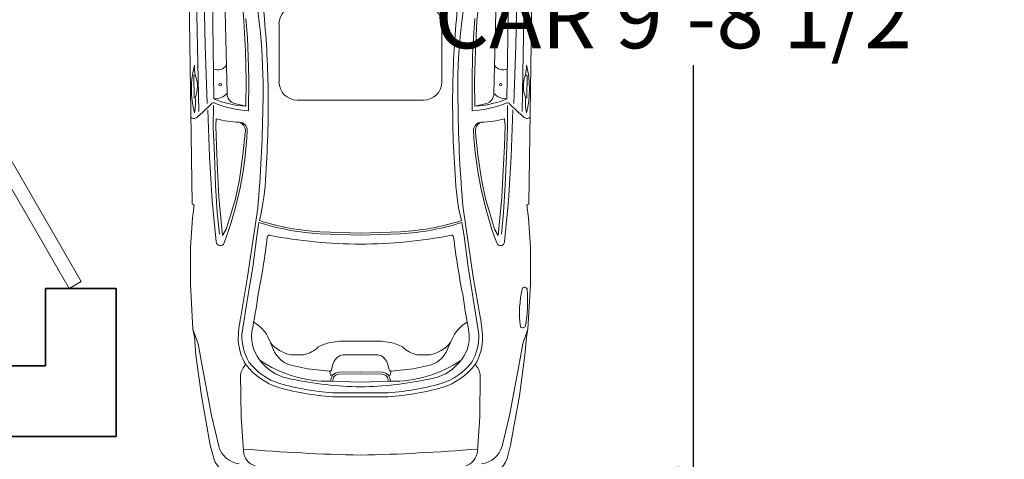
# Model space of a CAD drawing. Units: inches. Extents: x 2558 to 3026, y 433 to 1053.
# Tile 3 of 8: x 2795 to 2921, y 518 to 574. Entities that reach past the tile are written whole.
import ezdxf

# ---------------------------------------------------------------- set-up
doc = ezdxf.new("R2010")
doc.units = ezdxf.units.IN
for name, color, linetype, lineweight in [('0_Equip', 250, 'Continuous', 13), ('A-ANNO-DIMS', 2, 'Continuous', 18), ('A-DOOR', 4, 'Continuous', 18), ('A-WALL', 7, 'Continuous', 35)]:
    doc.layers.add(name, color=color, linetype=linetype, lineweight=lineweight)
doc.styles.get("Standard").update_dxf_attribs({"font": 'arial.ttf'})
doc.dimstyles.new('ISO-25', dxfattribs={"dimtxt": 8, "dimasz": 4, "dimexe": 1, "dimexo": 1, "dimgap": 1, "dimtad": 0, "dimtih": 1, "dimtoh": 1, "dimlunit": 3, "dimtxsty": 'Standard', "dimblk": 'OBLIQUE', "dimcen": 2.5, "dimclrt": 1, "dimadec": 0, "dimazin": 0, "dimtfac": 1, "dimtmove": 0, "dimatfit": 3, "dimfxl": 1, "dimfxlon": 1, "dimarcsym": 0})

# ---------------------------------------------------------------- blocks, each defined once
blk = doc.blocks.new('*U8')
for p, q in [((0, 0), (0, -6)), ((36, 0), (36, -6))]:
    blk.add_line(p, q)
blk.add_lwpolyline([(0, 0), (31.18, 18), (32.05, 16.48), (0.87, -1.52)], close=True)
blk.add_arc((0, 0), 36, 0, 30)
blk = doc.blocks.new('A$C4C7B54D1')
at = {"layer": '0_Equip', "ltscale": 0.1}
for p, q in [((-1.6171, 0.8152), (-1.5964, -0.6171)), ((-1.5805, 0.8299), (-1.5623, -0.138)), ((-1.4835, -0.0735), (-1.497, 0.863)), ((0.0322, -0.0735), (0.0457, 0.863)), ((0.1292, 0.8299), (0.111, -0.138)), ((0.1658, 0.8152), (0.145, -0.6171)), ((-1.4352, 0.792), (-1.4152, -0.045)), ((-0.0162, 0.792), (-0.0361, -0.045)), ((-1.5355, 0.484), (-1.5292, 0.2045)), ((0.0842, 0.484), (0.0779, 0.2045)), ((-1.3321, 0.3749), (-1.3286, 0.3301)), ((-0.1192, 0.3749), (-0.1228, 0.3301)), ((-1.3286, 0.3301), (-1.3204, 0.1751)), ((-1.3178, 0.3418), (-1.31, 0.2426)), ((-1.1468, 0.3145), (-1.1468, 0.0145)), ((-0.3045, 0.3145), (-0.3045, 0.0145)), ((-0.1335, 0.3418), (-0.1413, 0.2426)), ((-0.1228, 0.3301), (-0.1309, 0.1751)), ((-1.5292, 0.2045), (-1.5185, -0.0974)), ((-1.31, 0.2426), (-1.306, 0.1454)), ((-0.1413, 0.2426), (-0.1454, 0.1454)), ((0.0779, 0.2045), (0.0672, -0.0974)), ((-1.3204, 0.1751), (-1.3164, 0.0193)), ((-0.1309, 0.1751), (-0.1349, 0.0193)), ((-1.306, 0.1454), (-1.3036, 0.0305)), ((-0.1454, 0.1454), (-0.1478, 0.0305)), ((-1.5798, 0.0505), (-1.5879, 0.0456)), ((-1.5879, 0.0456), (-1.5863, -0.0676)), ((-1.3164, 0.0193), (-1.3178, -0.1112)), ((-1.3036, 0.0305), (-1.3044, -0.1358)), ((-0.1478, 0.0305), (-0.147, -0.1358)), ((-0.1349, 0.0193), (-0.1335, -0.1112)), ((0.1285, 0.0505), (0.1365, 0.0456)), ((0.1365, 0.0456), (0.1349, -0.0676)), ((-1.5863, -0.0676), (-1.5806, -0.0692)), ((-1.4948, -0.0965), (-1.5413, -0.143)), ((-1.3774, -0.0972), (-1.3178, -0.1112)), ((-0.7257, -0.0796), (-1.0528, -0.0796)), ((-0.7257, -0.0796), (-0.3986, -0.0796)), ((-0.0739, -0.0972), (-0.1335, -0.1112)), ((0.0435, -0.0965), (0.0899, -0.143)), ((0.1349, -0.0676), (0.1293, -0.0692)), ((-1.5413, -0.143), (-1.5686, -0.1663)), ((-1.5147, -0.1299), (-1.5058, -0.3725)), ((-1.4857, -0.1082), (-1.4866, -0.2223)), ((0.0344, -0.1082), (0.0352, -0.2223)), ((0.0633, -0.1299), (0.0545, -0.3725)), ((0.0899, -0.143), (0.1172, -0.1663)), ((-1.4713, -0.1773), (-1.4737, -0.2127)), ((0.02, -0.1773), (0.0224, -0.2127)), ((-1.4866, -0.2223), (-1.4809, -0.3653)), ((-1.4737, -0.2127), (-1.4705, -0.3187)), ((-1.3211, -0.2496), (-1.3332, -0.3629)), ((-0.1302, -0.2496), (-0.1182, -0.3629)), ((0.0224, -0.2127), (0.0192, -0.3187)), ((0.0352, -0.2223), (0.0296, -0.3653)), ((-1.4705, -0.3187), (-1.4649, -0.4424)), ((0.0192, -0.3187), (0.0135, -0.4424)), ((-1.5058, -0.3725), (-1.4922, -0.6007)), ((-1.4809, -0.3653), (-1.4745, -0.5203)), ((-1.3332, -0.3629), (-1.3516, -0.4906)), ((-0.1182, -0.3629), (-0.0997, -0.4906)), ((0.0296, -0.3653), (0.0232, -0.5203)), ((0.0545, -0.3725), (0.0408, -0.6007)), ((-1.4649, -0.4424), (-1.4576, -0.5822)), ((0.0135, -0.4424), (0.0063, -0.5822)), ((-1.3516, -0.4906), (-1.3725, -0.5902)), ((-0.0997, -0.4906), (-0.0788, -0.5902)), ((-1.4745, -0.5203), (-1.4665, -0.6617)), ((0.0232, -0.5203), (0.0151, -0.6617)), ((-1.4922, -0.6007), (-1.4712, -0.814)), ((-1.4576, -0.5822), (-1.4384, -0.7806)), ((-1.3725, -0.5902), (-1.3942, -0.6641)), ((-0.0788, -0.5902), (-0.0571, -0.6641)), ((0.0063, -0.5822), (-0.013, -0.7806)), ((0.0408, -0.6007), (0.0198, -0.814)), ((-1.5964, -0.6171), (-1.5863, -0.6228)), ((-1.5863, -0.6228), (-1.5949, -0.6885)), ((-1.4665, -0.6617), (-1.4552, -0.7742)), ((-1.3094, -0.9936), (-1.2569, -0.6398)), ((-0.1419, -0.9936), (-0.1944, -0.6398)), ((0.0151, -0.6617), (0.0039, -0.7742)), ((0.145, -0.6171), (0.1349, -0.6228)), ((0.1349, -0.6228), (0.1436, -0.6885)), ((-1.5949, -0.6885), (-1.605, -0.843)), ((-1.3942, -0.6641), (-1.4199, -0.7485)), ((-0.0571, -0.6641), (-0.0314, -0.7485)), ((0.1436, -0.6885), (0.1537, -0.843)), ((-1.4199, -0.7485), (-1.4384, -0.7806)), ((-1.2616, -0.7846), (-1.2511, -0.7134)), ((-0.9331, -0.7613), (-0.7253, -0.7683)), ((-0.5182, -0.7613), (-0.726, -0.7683)), ((-0.1898, -0.7846), (-0.2003, -0.7134)), ((-0.0314, -0.7485), (-0.013, -0.7806)), ((-1.2826, -0.9445), (-1.2616, -0.7846)), ((-0.9336, -0.7717), (-0.7257, -0.7787)), ((-0.5177, -0.7717), (-0.7257, -0.7787)), ((-0.1688, -0.9445), (-0.1898, -0.7846)), ((-1.605, -0.843), (-1.605, -1.0322)), ((0.1537, -0.843), (0.1537, -1.0322)), ((-1.3094, -1.1068), (-1.2826, -0.9445)), ((-0.1419, -1.1068), (-0.1688, -0.9445)), ((-1.3444, -1.2014), (-1.3094, -0.9936)), ((-0.1069, -1.2014), (-0.1419, -0.9936)), ((-1.605, -1.0322), (-1.592, -1.2661)), ((0.1537, -1.0322), (0.1407, -1.2661)), ((-1.3386, -1.2925), (-1.3094, -1.1068)), ((-0.1127, -1.2925), (-0.1419, -1.1068)), ((-1.565, -1.3405), (-1.592, -1.2661)), ((-1.592, -1.2661), (-1.5848, -1.3051)), ((0.1137, -1.3405), (0.1407, -1.2661)), ((0.1407, -1.2661), (0.1335, -1.3051)), ((-1.5848, -1.3051), (-1.5762, -1.4004)), ((-1.1985, -1.3182), (-1.1694, -1.3835)), ((-0.2528, -1.3182), (-0.282, -1.3835)), ((0.1335, -1.3051), (0.1248, -1.4004)), ((-1.5417, -1.4736), (-1.565, -1.3405)), ((-0.88, -1.3337), (-0.8328, -1.3271)), ((-0.8328, -1.3271), (-0.7257, -1.3271)), ((-0.6185, -1.3271), (-0.7257, -1.3271)), ((-0.5713, -1.3337), (-0.6185, -1.3271)), ((0.0904, -1.4736), (0.1137, -1.3405)), ((-1.5762, -1.4004), (-1.5486, -1.6107)), ((-1.0858, -1.3979), (-1.0181, -1.3979)), ((-0.8558, -1.4236), (-0.861, -1.4312)), ((-0.8488, -1.4158), (-0.8558, -1.4236)), ((-0.8409, -1.4088), (-0.8488, -1.4158)), ((-0.8309, -1.402), (-0.8409, -1.4088)), ((-0.8163, -1.3979), (-0.8309, -1.402)), ((-0.7257, -1.3974), (-0.8163, -1.3979)), ((-0.7257, -1.3974), (-0.635, -1.3979)), ((-0.635, -1.3979), (-0.6204, -1.402)), ((-0.6204, -1.402), (-0.6104, -1.4088)), ((-0.6104, -1.4088), (-0.6025, -1.4158)), ((-0.6025, -1.4158), (-0.5955, -1.4236)), ((-0.5955, -1.4236), (-0.5904, -1.4312)), ((-0.3655, -1.3979), (-0.4333, -1.3979)), ((0.1248, -1.4004), (0.0973, -1.6107)), ((-1.4962, -1.7129), (-1.5417, -1.4736)), ((-1.0923, -1.4501), (-0.9989, -1.4699)), ((-0.9989, -1.4699), (-0.8846, -1.4828)), ((-0.8745, -1.477), (-0.8769, -1.4791)), ((-0.8731, -1.467), (-0.8745, -1.477)), ((-0.8696, -1.4545), (-0.8731, -1.467)), ((-0.8664, -1.4423), (-0.8696, -1.4545)), ((-0.861, -1.4312), (-0.8664, -1.4423)), ((-0.5904, -1.4312), (-0.585, -1.4423)), ((-0.585, -1.4423), (-0.5817, -1.4545)), ((-0.5817, -1.4545), (-0.5782, -1.467)), ((-0.5782, -1.467), (-0.5768, -1.477)), ((-0.5768, -1.477), (-0.5744, -1.4791)), ((-0.4524, -1.4699), (-0.5668, -1.4828)), ((-0.359, -1.4501), (-0.4524, -1.4699)), ((0.0448, -1.7129), (0.0904, -1.4736)), ((-1.3456, -1.5004), (-1.3433, -1.7188)), ((-0.8807, -1.4821), (-0.8846, -1.4828)), ((-0.8846, -1.4828), (-0.8799, -1.5038)), ((-0.8769, -1.4791), (-0.8807, -1.4821)), ((-0.8799, -1.5038), (-0.8706, -1.5038)), ((-0.7257, -1.4865), (-0.8374, -1.4884)), ((-0.7257, -1.4969), (-0.837, -1.4988)), ((-0.7257, -1.4865), (-0.6139, -1.4884)), ((-0.7257, -1.4969), (-0.6143, -1.4988)), ((-0.5714, -1.5038), (-0.5808, -1.5038)), ((-0.5744, -1.4791), (-0.5706, -1.4821)), ((-0.5668, -1.4828), (-0.5714, -1.5038)), ((-0.5706, -1.4821), (-0.5668, -1.4828)), ((-0.1057, -1.5004), (-0.1081, -1.7188)), ((-0.8799, -1.5352), (-0.7257, -1.5393)), ((-0.5714, -1.5352), (-0.7257, -1.5393)), ((-1.5486, -1.6107), (-1.5024, -1.8663)), ((-0.8507, -1.616), (-0.7257, -1.616)), ((-0.8502, -1.5951), (-0.7257, -1.5951)), ((-0.6011, -1.5951), (-0.7257, -1.5951)), ((-0.6006, -1.616), (-0.7257, -1.616)), ((0.0973, -1.6107), (0.0511, -1.8663)), ((-1.4584, -1.8701), (-1.4962, -1.7129)), ((-1.3433, -1.7188), (-1.3304, -1.8962)), ((-0.1081, -1.7188), (-0.1209, -1.8962)), ((0.0071, -1.8701), (0.0448, -1.7129)), ((-1.5024, -1.8663), (-1.4894, -1.914)), ((0.0511, -1.8663), (0.0381, -1.914))]:
    blk.add_line(p, q, dxfattribs=at)
for centre in [(-1.4513, 0), (0, 0)]:
    blk.add_circle(centre, 0.00662, dxfattribs=at)
for centre, radius, start, end in [((-4.2099, -0.0242), 2.9809, 358.1905, 11.4064), ((2.7585, -0.0242), 2.9809, 168.5936, 181.8095), ((-6.5594, -0.126), 5.3575, 1.3159, 5.7952), ((-1.0528, 0.3145), 0.0941, 90, 180), ((-0.3986, 0.3145), 0.0941, 0, 90), ((5.1081, -0.126), 5.3575, 174.2048, 178.6841), ((-1.0944, -0.0222), 0.5055, 165.8807, 194.1193), ((-1.3066, 0.102), 0.2781, 180.1936, 190.6834), ((-1.4634, 0.1296), 0.0534, 245.2796, 326.9469), ((0.0121, 0.1296), 0.0534, 213.0531, 294.7204), ((-0.1448, 0.102), 0.2781, 349.3166, 359.8064), ((-0.3569, -0.0222), 0.5055, 345.8807, 14.1193), ((-1.7275, -0.0084), 0.159, 337.4976, 21.7335), ((-1.0528, 0.0145), 0.0941, 180, 270), ((-0.3986, 0.0145), 0.0941, 270, 0), ((0.2762, -0.0084), 0.159, 158.2665, 202.5024), ((-1.4831, 0.0214), 0.095, 269.7172, 315.6185), ((-1.3634, -0.0473), 0.0519, 177.4537, 254.2676), ((-6.573, -0.0941), 5.3705, 356.0501, 0.9723), ((5.1217, -0.0941), 5.3705, 179.0277, 183.9499), ((-0.0879, -0.0473), 0.0519, 285.7324, 2.5463), ((0.0317, 0.0214), 0.095, 224.3815, 270.2828), ((-1.7817, -0.0969), 0.2029, 346.1346, 7.8419), ((-1.4874, -0.1039), 0.0105, 68.8598, 135.0096), ((-1.2476, 0.5164), 0.6547, 248.8598, 265.0222), ((-1.2968, 0.3651), 0.4767, 246.9385, 267.4714), ((-0.2038, 0.5164), 0.6547, 274.9778, 291.1402), ((-0.1545, 0.3651), 0.4767, 272.5286, 293.0615), ((0.0361, -0.1039), 0.0105, 44.9904, 111.1402), ((0.3303, -0.0969), 0.2029, 172.1581, 193.8654), ((-8.0298, -0.0355), 6.7998, 354.90123, 359.30214), ((6.5785, -0.0355), 6.7998, 180.69786, 185.09877), ((-1.5869, -0.1514), 0.0236, 227.2909, 320.7388), ((-1.3362, 0.3542), 0.5484, 255.7347, 268.4072), ((-1.3699, -0.2402), 0.0497, 349.0381, 68.1064), ((-1.3526, -0.2358), 0.0418, 357.143, 88.4072), ((-0.0988, -0.2358), 0.0418, 91.5928, 182.857), ((-0.0814, -0.2402), 0.0497, 111.8936, 190.9619), ((-0.1152, 0.3542), 0.5484, 271.5928, 284.2653), ((0.1355, -0.1514), 0.0236, 219.2612, 312.7091), ((-3.2483, -0.1412), 1.9399, 339.54, 357.143), ((1.797, -0.1412), 1.9399, 182.857, 200.46), ((-2.454, -0.4173), 1.2396, 346.6558, 357.8401), ((1.0027, -0.4173), 1.2396, 182.1599, 193.3442), ((-0.8588, 0.5276), 1.291, 252.4566, 266.6988), ((-0.5926, 0.5276), 1.291, 273.3012, 287.5434), ((-0.8588, 0.5276), 1.3014, 252.4566, 266.7043), ((-0.5926, 0.5276), 1.3014, 273.2957, 287.5434), ((-1.4504, -0.812), 0.0209, 185.6259, 339.54), ((-5.088, -0.3237), 3.9082, 348.7726, 353.1671), ((-1.1971, -0.7899), 0.0105, 79.1189, 173.1671), ((-0.7142, 1.7227), 2.5481, 259.1189, 269.7413), ((-0.7372, 1.7227), 2.5481, 270.2587, 280.8811), ((-0.2542, -0.7899), 0.0105, 6.8329, 100.8811), ((3.6366, -0.3237), 3.9082, 186.8329, 191.2274), ((-0.001, -0.812), 0.0209, 200.46, 354.3741), ((0.625, -1.1812), 0.5281, 165.7822, 187.813), ((0.1224, -1.0639), 0.0155, 11.61, 127.0083), ((-0.7003, -1.1122), 0.8395, 350.5693, 3.5107), ((-4.7286, -0.6026), 3.5073, 348.8701, 352.1003), ((3.2772, -0.6026), 3.5073, 187.8997, 191.1299), ((-0.8187, -1.3185), 0.5386, 167.4447, 180.7102), ((-0.6326, -1.3185), 0.5386, 359.2898, 12.5553), ((-1.3591, -1.3822), 0.1728, 21.7432, 61.9432), ((-0.0922, -1.3822), 0.1728, 118.0568, 158.2568), ((0.1138, -1.243), 0.0156, 219.7819, 334.4738), ((-1.0611, -1.2979), 0.2775, 178.8811, 209.7062), ((-1.0952, -1.3051), 0.1937, 172.4314, 224.4267), ((-0.3561, -1.3051), 0.1937, 315.5733, 7.5686), ((-0.3902, -1.2979), 0.2775, 330.2938, 1.1189), ((-1.0944, -1.3104), 0.2633, 183.2136, 211.504), ((-1.0482, -1.2146), 0.1871, 220.4031, 258.3959), ((-1.0495, -1.2507), 0.1505, 282.0448, 314.7653), ((-0.8301, -1.5634), 0.235, 102.268, 118.8572), ((-0.6213, -1.5634), 0.235, 61.1428, 77.732), ((-0.4019, -1.2507), 0.1505, 225.2347, 257.9552), ((-0.4032, -1.2146), 0.1871, 281.6041, 319.5969), ((-0.3569, -1.3104), 0.2633, 328.496, 356.7864), ((-1.0421, -1.3141), 0.145, 208.6187, 249.7318), ((-0.4092, -1.3141), 0.145, 290.2682, 331.3813), ((-1.2501, -1.516), 0.0967, 135.2951, 170.7274), ((-1.052, -1.2472), 0.3339, 216.9484, 253.2314), ((-1.052, -1.2472), 0.313, 216.9484, 253.2054), ((-0.8912, -0.9022), 0.6331, 235.8724, 271.0227), ((-1.0459, -1.2776), 0.2487, 221.0065, 261.6946), ((-0.5601, -0.9022), 0.6331, 268.9773, 304.1276), ((-0.4054, -1.2776), 0.2487, 278.3054, 318.9935), ((-0.3993, -1.2472), 0.313, 286.7946, 323.0516), ((-0.3993, -1.2472), 0.3339, 286.7686, 323.0516), ((-0.2012, -1.516), 0.0967, 9.2726, 44.7049), ((-0.7003, 0.2815), 1.8451, 258.0669, 269.2129), ((-0.8066, -1.54), 0.0735, 150.5285, 176.2825), ((-0.8344, -1.538), 0.0498, 93.4455, 136.5439), ((-0.8066, -1.54), 0.063, 151.7195, 175.9212), ((-0.8344, -1.538), 0.0393, 93.7549, 134.7116), ((-0.751, 0.2815), 1.8451, 270.7871, 281.9331), ((-0.6169, -1.538), 0.0393, 45.2884, 86.2451), ((-0.6169, -1.538), 0.0498, 43.4561, 86.5545), ((-0.6447, -1.54), 0.063, 4.0788, 28.2805), ((-0.6447, -1.54), 0.0735, 3.7175, 29.4715), ((-0.7884, -0.3101), 1.3074, 254.0198, 267.2681), ((-0.7884, -0.3101), 1.2865, 254.0263, 267.246), ((-0.6629, -0.3101), 1.2865, 272.754, 285.9737), ((-0.6629, -0.3101), 1.3074, 272.7319, 285.9802), ((-1.3393, -1.8393), 0.123, 194.4986, 263.7836), ((-0.1121, -1.8393), 0.123, 276.2164, 345.5014), ((-1.3628, -1.8937), 0.1282, 189.093, 262.4153), ((-0.5134, 7.9307), 9.8503, 265.23745, 268.76503), ((-1.2452, -1.8915), 0.0853, 183.2055, 252.6405), ((-0.938, 7.9307), 9.8503, 271.23497, 274.76255), ((-0.2061, -1.8915), 0.0853, 287.3595, 356.7945), ((-0.0885, -1.8937), 0.1282, 277.5847, 350.907)]:
    blk.add_arc(centre, radius, start, end, dxfattribs=at)
blk = doc.blocks.new('_Oblique')
at = {"color": 0, "linetype": 'ByBlock', "lineweight": -2}
blk.add_line((-0.5, -0.5), (0.5, 0.5), dxfattribs=at)
blk = doc.blocks.new('*D43')
at = {"layer": 'A-ANNO-DIMS', "color": 0, "lineweight": -2, "transparency": 16777216}
for p, q in [((2880.07, 631.47), (2882.07, 631.47)), ((2881.07, 631.47), (2881.07, 578.35)), ((2881.07, 514.96), (2881.07, 568.08)), ((2880.07, 514.96), (2882.07, 514.96))]:
    blk.add_line(p, q, dxfattribs=at)
at = {"layer": 'Defpoints', "color": 0, "transparency": 16777216}
for p in [(2863.59, 631.47), (2881.07, 631.47), (2863.59, 514.96)]:
    blk.add_point(p, dxfattribs=at)
at = {"layer": 'A-ANNO-DIMS', "color": 0, "lineweight": -2, "transparency": 16777216, "xscale": 4, "yscale": 4, "zscale": 4}
for p, rotation in [((2881.07, 631.47), 90), ((2881.07, 514.96), 270)]:
    blk.add_blockref('_Oblique', p, dxfattribs=dict(at, rotation=rotation))
at = {"layer": 'A-ANNO-DIMS', "color": 1, "transparency": 16777216, "insert": (2881.07, 573.21), "char_height": 8, "attachment_point": 5}
blk.add_mtext('CAR 9\'-8 1/2"', dxfattribs=at)
blk = doc.blocks.new('*D45')
at = {"layer": 'A-ANNO-DIMS', "color": 0, "lineweight": -2, "transparency": 16777216}
for p, q in [((2803.13, 445.87), (2803.13, 443.87)), ((2803.13, 444.87), (2831.63, 444.87)), ((2831.63, 445.87), (2831.63, 443.87)), ((2831.63, 444.87), (2835.63, 444.87))]:
    blk.add_line(p, q, dxfattribs=at)
at = {"layer": 'Defpoints', "color": 0, "transparency": 16777216}
for p in [(2803.13, 799.82), (2831.63, 799.82), (2831.63, 444.87)]:
    blk.add_point(p, dxfattribs=at)
at = {"layer": 'A-ANNO-DIMS', "color": 0, "lineweight": -2, "transparency": 16777216, "xscale": 4, "yscale": 4, "zscale": 4, "rotation": 180}
blk.add_blockref('_Oblique', (2803.13, 444.87), dxfattribs=at)
at = {"layer": 'A-ANNO-DIMS', "color": 0, "lineweight": -2, "transparency": 16777216, "xscale": 4, "yscale": 4, "zscale": 4}
blk.add_blockref('_Oblique', (2831.63, 444.87), dxfattribs=at)
at = {"layer": 'A-ANNO-DIMS', "color": 1, "transparency": 16777216, "insert": (2856.65, 444.87), "char_height": 8, "attachment_point": 5}
blk.add_mtext('2\'-4 1/2"', dxfattribs=at)
blk = doc.blocks.new('*D49')
at = {"layer": 'A-ANNO-DIMS', "color": 0, "lineweight": -2, "transparency": 16777216}
for p, q in [((2839.13, 445.87), (2839.13, 443.87)), ((2839.13, 444.87), (2845.5, 444.87)), ((2875.13, 444.87), (2868.76, 444.87)), ((2875.13, 445.87), (2875.13, 443.87))]:
    blk.add_line(p, q, dxfattribs=at)
at = {"layer": 'Defpoints', "color": 0, "transparency": 16777216}
for p in [(2839.13, 790.82), (2875.13, 790.82), (2875.13, 444.87)]:
    blk.add_point(p, dxfattribs=at)
at = {"layer": 'A-ANNO-DIMS', "color": 0, "lineweight": -2, "transparency": 16777216, "xscale": 4, "yscale": 4, "zscale": 4, "rotation": 180}
blk.add_blockref('_Oblique', (2839.13, 444.87), dxfattribs=at)
at = {"layer": 'A-ANNO-DIMS', "color": 0, "lineweight": -2, "transparency": 16777216, "xscale": 4, "yscale": 4, "zscale": 4}
blk.add_blockref('_Oblique', (2875.13, 444.87), dxfattribs=at)
at = {"layer": 'A-ANNO-DIMS', "color": 1, "transparency": 16777216, "insert": (2857.13, 444.87), "char_height": 8, "attachment_point": 5}
blk.add_mtext('3\'-0"', dxfattribs=at)
blk = doc.blocks.new('*D50')
at = {"layer": 'A-ANNO-DIMS', "color": 0, "lineweight": -2, "transparency": 16777216}
for p, q in [((2807.63, 445.87), (2807.63, 443.87)), ((2807.63, 444.87), (2826, 444.87)), ((2867.63, 444.87), (2849.27, 444.87)), ((2867.63, 445.87), (2867.63, 443.87))]:
    blk.add_line(p, q, dxfattribs=at)
at = {"layer": 'Defpoints', "color": 0, "transparency": 16777216}
for p in [(2807.63, 649.82), (2867.63, 649.82), (2867.63, 444.87)]:
    blk.add_point(p, dxfattribs=at)
at = {"layer": 'A-ANNO-DIMS', "color": 0, "lineweight": -2, "transparency": 16777216, "xscale": 4, "yscale": 4, "zscale": 4, "rotation": 180}
blk.add_blockref('_Oblique', (2807.63, 444.87), dxfattribs=at)
at = {"layer": 'A-ANNO-DIMS', "color": 0, "lineweight": -2, "transparency": 16777216, "xscale": 4, "yscale": 4, "zscale": 4}
blk.add_blockref('_Oblique', (2867.63, 444.87), dxfattribs=at)
at = {"layer": 'A-ANNO-DIMS', "color": 1, "transparency": 16777216, "insert": (2837.63, 444.87), "char_height": 8, "attachment_point": 5}
blk.add_mtext('5\'-0"', dxfattribs=at)
blk = doc.blocks.new('*D60')
at = {"layer": 'A-ANNO-DIMS', "color": 0, "lineweight": -2, "transparency": 16777216}
for p, q in [((2996.58, 575.69), (2998.58, 575.69)), ((2997.58, 575.69), (2997.58, 562.78)), ((2997.58, 539.69), (2997.58, 552.6)), ((2996.58, 539.69), (2998.58, 539.69))]:
    blk.add_line(p, q, dxfattribs=at)
at = {"layer": 'Defpoints', "color": 0, "transparency": 16777216}
for p in [(2807.63, 575.69), (2997.58, 575.69), (2807.63, 539.69)]:
    blk.add_point(p, dxfattribs=at)
at = {"layer": 'A-ANNO-DIMS', "color": 0, "lineweight": -2, "transparency": 16777216, "xscale": 4, "yscale": 4, "zscale": 4}
for p, rotation in [((2997.58, 575.69), 90), ((2997.58, 539.69), 270)]:
    blk.add_blockref('_Oblique', p, dxfattribs=dict(at, rotation=rotation))
at = {"layer": 'A-ANNO-DIMS', "color": 1, "transparency": 16777216, "insert": (2997.58, 557.69), "char_height": 8, "attachment_point": 5}
blk.add_mtext('3\'-0"', dxfattribs=at)
blk = doc.blocks.new('*D63')
at = {"layer": 'A-ANNO-DIMS', "color": 0, "lineweight": -2, "transparency": 16777216}
for p, q in [((2757.89, 445.87), (2757.89, 443.87)), ((2757.89, 444.87), (2765.63, 444.87)), ((2765.63, 445.87), (2765.63, 443.87)), ((2765.63, 444.87), (2769.63, 444.87))]:
    blk.add_line(p, q, dxfattribs=at)
at = {"layer": 'Defpoints', "color": 0, "transparency": 16777216}
for p in [(2757.89, 943.82), (2765.63, 943.82), (2765.63, 444.87)]:
    blk.add_point(p, dxfattribs=at)
at = {"layer": 'A-ANNO-DIMS', "color": 0, "lineweight": -2, "transparency": 16777216, "xscale": 4, "yscale": 4, "zscale": 4, "rotation": 180}
blk.add_blockref('_Oblique', (2757.89, 444.87), dxfattribs=at)
at = {"layer": 'A-ANNO-DIMS', "color": 0, "lineweight": -2, "transparency": 16777216, "xscale": 4, "yscale": 4, "zscale": 4}
blk.add_blockref('_Oblique', (2765.63, 444.87), dxfattribs=at)
at = {"layer": 'A-ANNO-DIMS', "color": 1, "transparency": 16777216, "insert": (2790.59, 444.87), "char_height": 8, "attachment_point": 5}
blk.add_mtext('0\'-7 1/2"', dxfattribs=at)
blk = doc.blocks.new('*D69')
at = {"layer": 'A-ANNO-DIMS', "color": 0, "lineweight": -2, "transparency": 16777216}
for p, q in [((2790.04, 445.87), (2790.04, 443.87)), ((2790.04, 444.87), (2807.63, 444.87)), ((2807.63, 445.87), (2807.63, 443.87)), ((2807.63, 444.87), (2811.63, 444.87))]:
    blk.add_line(p, q, dxfattribs=at)
at = {"layer": 'Defpoints', "color": 0, "transparency": 16777216}
for p in [(2790.04, 520.82), (2807.63, 520.82), (2807.63, 444.87)]:
    blk.add_point(p, dxfattribs=at)
at = {"layer": 'A-ANNO-DIMS', "color": 0, "lineweight": -2, "transparency": 16777216, "xscale": 4, "yscale": 4, "zscale": 4, "rotation": 180}
blk.add_blockref('_Oblique', (2790.04, 444.87), dxfattribs=at)
at = {"layer": 'A-ANNO-DIMS', "color": 0, "lineweight": -2, "transparency": 16777216, "xscale": 4, "yscale": 4, "zscale": 4}
blk.add_blockref('_Oblique', (2807.63, 444.87), dxfattribs=at)
at = {"layer": 'A-ANNO-DIMS', "color": 1, "transparency": 16777216, "insert": (2832.21, 444.87), "char_height": 8, "attachment_point": 5}
blk.add_mtext('1\'-5 1/2"', dxfattribs=at)
blk = doc.blocks.new('*D71')
at = {"layer": 'A-ANNO-DIMS', "color": 0, "lineweight": -2, "transparency": 16777216}
for p, q in [((2996.58, 539.69), (2998.58, 539.69)), ((2997.58, 539.69), (2997.58, 535.27)), ((2997.58, 520.82), (2997.58, 525.24)), ((2996.58, 520.82), (2998.58, 520.82))]:
    blk.add_line(p, q, dxfattribs=at)
at = {"layer": 'Defpoints', "color": 0, "transparency": 16777216}
for p in [(2807.63, 539.69), (2997.58, 539.69), (2807.63, 520.82)]:
    blk.add_point(p, dxfattribs=at)
at = {"layer": 'A-ANNO-DIMS', "color": 0, "lineweight": -2, "transparency": 16777216, "xscale": 4, "yscale": 4, "zscale": 4}
for p, rotation in [((2997.58, 539.69), 90), ((2997.58, 520.82), 270)]:
    blk.add_blockref('_Oblique', p, dxfattribs=dict(at, rotation=rotation))
at = {"layer": 'A-ANNO-DIMS', "color": 1, "transparency": 16777216, "insert": (2997.58, 530.26), "char_height": 8, "attachment_point": 5}
blk.add_mtext('1\'-7"', dxfattribs=at)
blk = doc.blocks.new('*D73')
at = {"layer": 'A-ANNO-DIMS', "color": 0, "lineweight": -2, "transparency": 16777216}
for p, q in [((2816.63, 1039.77), (2816.63, 1041.77)), ((2959.63, 1039.77), (2959.63, 1041.77)), ((2816.63, 1040.77), (2870.66, 1040.77)), ((2959.63, 1040.77), (2905.6, 1040.77))]:
    blk.add_line(p, q, dxfattribs=at)
at = {"layer": 'Defpoints', "color": 0, "transparency": 16777216}
for p in [(2959.63, 1040.77), (2816.63, 481.83), (2959.63, 481.82)]:
    blk.add_point(p, dxfattribs=at)
at = {"layer": 'A-ANNO-DIMS', "color": 0, "lineweight": -2, "transparency": 16777216, "xscale": 4, "yscale": 4, "zscale": 4, "rotation": 180}
blk.add_blockref('_Oblique', (2816.63, 1040.77), dxfattribs=at)
at = {"layer": 'A-ANNO-DIMS', "color": 0, "lineweight": -2, "transparency": 16777216, "xscale": 4, "yscale": 4, "zscale": 4}
blk.add_blockref('_Oblique', (2959.63, 1040.77), dxfattribs=at)
at = {"layer": 'A-ANNO-DIMS', "color": 1, "transparency": 16777216, "insert": (2888.13, 1040.77), "char_height": 8, "attachment_point": 5}
blk.add_mtext('11\'-11"', dxfattribs=at)
blk = doc.blocks.new('*D75')
at = {"layer": 'A-ANNO-DIMS', "color": 0, "lineweight": -2, "transparency": 16777216}
for p, q in [((2831.63, 445.87), (2831.63, 443.87)), ((2831.63, 444.87), (2839.13, 444.87)), ((2839.13, 445.87), (2839.13, 443.87)), ((2839.13, 444.87), (2843.13, 444.87))]:
    blk.add_line(p, q, dxfattribs=at)
at = {"layer": 'Defpoints', "color": 0, "transparency": 16777216}
for p in [(2831.63, 799.82), (2839.13, 799.82), (2839.13, 444.87)]:
    blk.add_point(p, dxfattribs=at)
at = {"layer": 'A-ANNO-DIMS', "color": 0, "lineweight": -2, "transparency": 16777216, "xscale": 4, "yscale": 4, "zscale": 4, "rotation": 180}
blk.add_blockref('_Oblique', (2831.63, 444.87), dxfattribs=at)
at = {"layer": 'A-ANNO-DIMS', "color": 0, "lineweight": -2, "transparency": 16777216, "xscale": 4, "yscale": 4, "zscale": 4}
blk.add_blockref('_Oblique', (2839.13, 444.87), dxfattribs=at)
at = {"layer": 'A-ANNO-DIMS', "color": 1, "transparency": 16777216, "insert": (2864.09, 444.87), "char_height": 8, "attachment_point": 5}
blk.add_mtext('0\'-7 1/2"', dxfattribs=at)
blk = doc.blocks.new('*D76')
at = {"layer": 'A-ANNO-DIMS', "color": 0, "lineweight": -2, "transparency": 16777216}
for p, q in [((2879.03, 445.87), (2879.03, 443.87)), ((2879.03, 444.87), (2883.32, 444.87)), ((2911.03, 444.87), (2906.73, 444.87)), ((2911.03, 445.87), (2911.03, 443.87))]:
    blk.add_line(p, q, dxfattribs=at)
at = {"layer": 'Defpoints', "color": 0, "transparency": 16777216}
for p in [(2879.03, 943.82), (2911.03, 943.82), (2911.03, 444.87)]:
    blk.add_point(p, dxfattribs=at)
at = {"layer": 'A-ANNO-DIMS', "color": 0, "lineweight": -2, "transparency": 16777216, "xscale": 4, "yscale": 4, "zscale": 4, "rotation": 180}
blk.add_blockref('_Oblique', (2879.03, 444.87), dxfattribs=at)
at = {"layer": 'A-ANNO-DIMS', "color": 0, "lineweight": -2, "transparency": 16777216, "xscale": 4, "yscale": 4, "zscale": 4}
blk.add_blockref('_Oblique', (2911.03, 444.87), dxfattribs=at)
at = {"layer": 'A-ANNO-DIMS', "color": 1, "transparency": 16777216, "insert": (2895.03, 444.87), "char_height": 8, "attachment_point": 5}
blk.add_mtext('2\'-8"', dxfattribs=at)
blk = doc.blocks.new('*D77')
at = {"layer": 'A-ANNO-DIMS', "color": 0, "lineweight": -2, "transparency": 16777216}
for p, q in [((2867.63, 445.87), (2867.63, 443.87)), ((2867.63, 444.87), (2875.13, 444.87)), ((2875.13, 445.87), (2875.13, 443.87)), ((2875.13, 444.87), (2879.13, 444.87))]:
    blk.add_line(p, q, dxfattribs=at)
at = {"layer": 'Defpoints', "color": 0, "transparency": 16777216}
for p in [(2867.63, 658.82), (2875.13, 658.82), (2875.13, 444.87)]:
    blk.add_point(p, dxfattribs=at)
at = {"layer": 'A-ANNO-DIMS', "color": 0, "lineweight": -2, "transparency": 16777216, "xscale": 4, "yscale": 4, "zscale": 4, "rotation": 180}
blk.add_blockref('_Oblique', (2867.63, 444.87), dxfattribs=at)
at = {"layer": 'A-ANNO-DIMS', "color": 0, "lineweight": -2, "transparency": 16777216, "xscale": 4, "yscale": 4, "zscale": 4}
blk.add_blockref('_Oblique', (2875.13, 444.87), dxfattribs=at)
at = {"layer": 'A-ANNO-DIMS', "color": 1, "transparency": 16777216, "insert": (2900.09, 444.87), "char_height": 8, "attachment_point": 5}
blk.add_mtext('0\'-7 1/2"', dxfattribs=at)

msp = doc.modelspace()

# ---------------------------------------------------------------- linework, layer by layer
at = {"layer": 'A-WALL'}
for p, q in [((2798.633, 539.691), (2807.633, 539.691)), ((2798.633, 539.691), (2798.633, 529.825)), ((2807.633, 539.691), (2807.633, 520.825)), ((2798.633, 529.825), (2678.633, 529.825)), ((2807.633, 520.825), (2738.633, 520.825))]:
    msp.add_line(p, q, dxfattribs=at)

# ---------------------------------------------------------------- block references
at = {"layer": '0_Equip', "xscale": 24.59206405529848, "yscale": 24.59206405529848, "zscale": 24.59206405529848}
msp.add_blockref('A$C4C7B54D1', (2856.54, 565.611), dxfattribs=at)
at = {"layer": 'A-DOOR', "rotation": 90}
msp.add_blockref('*U8', (2801.633, 539.691), dxfattribs=at)

# ---------------------------------------------------------------- dimensions: what is measured, and where the dimension line sits
at = {"layer": 'A-ANNO-DIMS'}
for base, p1, p2, picture, middle in [((2959.633, 1040.775), (2816.633, 481.827), (2959.633, 481.825), '*D73', (2888.133, 1040.775)), ((2765.633, 444.875), (2757.892, 943.825), (2765.633, 943.825), '*D63', (2790.586, 444.875)), ((2911.025, 444.875), (2879.025, 943.825), (2911.025, 943.825), '*D76', (2895.025, 444.875)), ((2831.633, 444.875), (2803.133, 799.825), (2831.633, 799.825), '*D45', (2856.654, 444.875)), ((2839.133, 444.875), (2831.633, 799.825), (2839.133, 799.825), '*D75', (2864.086, 444.875)), ((2875.133, 444.875), (2839.133, 790.825), (2875.133, 790.825), '*D49', (2857.133, 444.875)), ((2875.133, 444.875), (2867.633, 658.825), (2875.133, 658.825), '*D77', (2900.086, 444.875)), ((2867.633, 444.875), (2807.633, 649.825), (2867.633, 649.825), '*D50', (2837.633, 444.875)), ((2807.633, 444.875), (2790.035, 520.825), (2807.633, 520.825), '*D69', (2832.21, 444.875))]:
    dim = msp.add_linear_dim(base=base, p1=p1, p2=p2, dimstyle='ISO-25', override={"dimdec": 1, "dimlfac": 1, "dimrnd": 0, "dimzin": 1, "dimdsep": 46, "dimlunit": 4, "dimfrac": 2}, dxfattribs=at)
    dim.commit()
    dim.dimension.update_dxf_attribs({"geometry": picture, "text_midpoint": middle})
dim = msp.add_linear_dim(base=(2881.069, 631.468), p1=(2863.592, 514.956), p2=(2863.592, 631.468), angle=90, text='CAR <>', dimstyle='ISO-25', override={"dimdec": 1, "dimlfac": 1, "dimrnd": 0, "dimzin": 1, "dimdsep": 46, "dimlunit": 4, "dimfrac": 2}, dxfattribs=at)
dim.commit()
dim.dimension.update_dxf_attribs({"geometry": '*D43', "text_midpoint": (2881.069, 573.212)})
for base, p1, p2, picture, middle in [((2997.583, 575.691), (2807.633, 539.691), (2807.633, 575.691), '*D60', (2997.583, 557.691)), ((2997.583, 539.691), (2807.633, 520.825), (2807.633, 539.691), '*D71', (2997.583, 530.258))]:
    dim = msp.add_linear_dim(base=base, p1=p1, p2=p2, angle=90, dimstyle='ISO-25', override={"dimdec": 1, "dimlfac": 1, "dimrnd": 0, "dimzin": 1, "dimdsep": 46, "dimlunit": 4, "dimfrac": 2}, dxfattribs=at)
    dim.commit()
    dim.dimension.update_dxf_attribs({"geometry": picture, "text_midpoint": middle})

doc.saveas('drawing.dxf')
